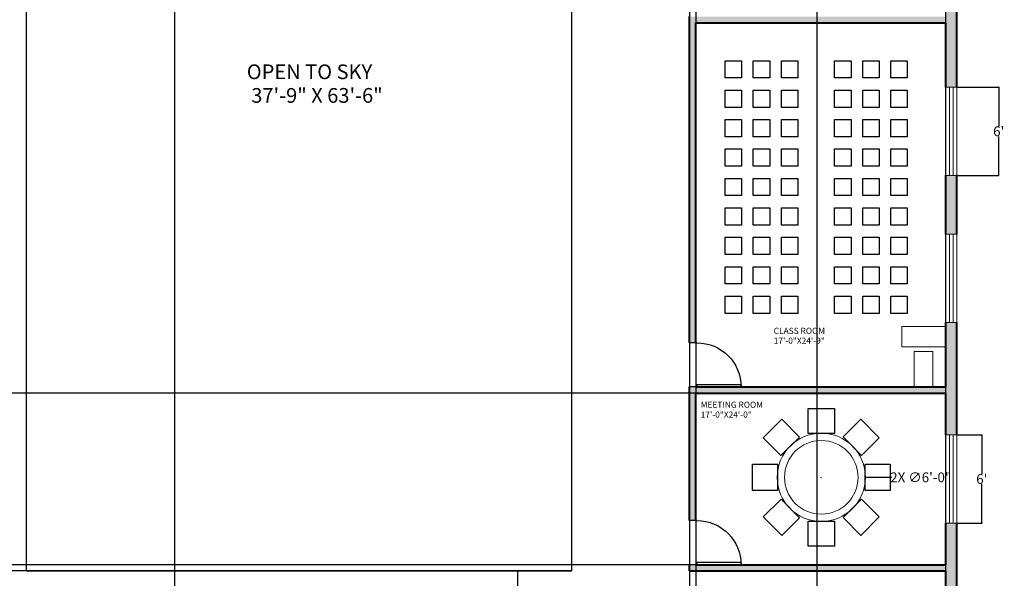
# Model space of a CAD drawing. Units: inches. Extents: x -405 to 940, y 226 to 2032.
# Tile 7 of 10: x 51 to 854, y 846 to 1301. Entities that reach past the tile are written whole.
import ezdxf

# ---------------------------------------------------------------- set-up
doc = ezdxf.new("R2010")
doc.units = ezdxf.units.IN
doc.header["$MEASUREMENT"] = 0
doc.linetypes.add('ACAD_ISO02W100', pattern=[15, 12, -3])
for name, color, linetype, lineweight in [('A-ANNO-DIMS', 120, 'Continuous', 18), ('A-AREA-IDEN', 32, 'Continuous', 18), ('A-FLOR-EDGE', 3, 'Continuous', 25), ('A-FURN-SEAT', 5, 'Continuous', 18), ('A-GLAZ-HIDN', 1, 'ACAD_ISO02W100', 18), ('A-WALL-PATT', 8, 'Continuous', 13), ('door', 6, 'Continuous', 25), ('tables', 2, 'Continuous', 18), ('wall', 3, 'Continuous', 40), ('window', 1, 'Continuous', 18)]:
    doc.layers.add(name, color=color, linetype=linetype, lineweight=lineweight)
doc.layers.add('beches', color=5, linetype='Continuous')
doc.styles.get("Standard").update_dxf_attribs({"font": 'arial.ttf'})
doc.dimstyles.get("Standard").update_dxf_attribs({"dimtxt": 8, "dimasz": 0.18, "dimexe": 0.18, "dimexo": 0.0625, "dimgap": 0.09, "dimtad": 0, "dimtih": 1, "dimtoh": 1, "dimdec": 0, "dimzin": 0, "dimdsep": 46, "dimlunit": 3, "dimtxsty": 'Standard', "dimblk": 'OBLIQUE', "dimcen": 0.09, "dimadec": 0, "dimazin": 0, "dimtfac": 1, "dimtdec": 0, "dimtofl": 0, "dimtmove": 0, "dimatfit": 3, "dimfxl": 1, "dimtolj": 1, "dimtzin": 0, "dimarcsym": 0})

# ---------------------------------------------------------------- blocks, each defined once
blk = doc.blocks.new('*U4')
for p, q in [((0, 0), (0, -6)), ((36, 0), (36, -6))]:
    blk.add_line(p, q)
blk.add_lwpolyline([(0, 0), (0, 36), (1.75, 36), (1.75, 0)], close=True)
blk.add_arc((0, 0), 36, 0, 90)
blk = doc.blocks.new('*U21')
at = {"layer": 'beches'}
blk.add_lwpolyline([(6.71, -7.02), (-6.71, -7.02), (-6.71, 7.02), (6.71, 7.02)], close=True, dxfattribs=at)
blk = doc.blocks.new('*U22')
at = {"layer": 'A-FURN-SEAT', "transparency": 16777216}
for p in [(-45.84, 192), (-45.84, 192, 12), (-45.84, 192, 24), (-45.84, 192, 36), (-45.84, 192, 48), (-45.84, 192, 60), (-45.84, 192, 72), (-45.84, 192, 84), (-45.84, 192, 96), (-45.84, 192, 108), (-45.84, 192, 120), (-45.84, 192, 132), (-22.92, 192), (-22.92, 192, 12), (-22.92, 192, 24), (-22.92, 192, 36), (-22.92, 192, 48), (-22.92, 192, 60), (-22.92, 192, 72), (-22.92, 192, 84), (-22.92, 192, 96), (-22.92, 192, 108), (-22.92, 192, 120), (-22.92, 192, 132), (0, 192), (0, 192, 12), (0, 192, 24), (0, 192, 36), (0, 192, 48), (0, 192, 60), (0, 192, 72), (0, 192, 84), (0, 192, 96), (0, 192, 108), (0, 192, 120), (0, 192, 132), (-45.84, 168), (-45.84, 168, 12), (-45.84, 168, 24), (-45.84, 168, 36), (-45.84, 168, 48), (-45.84, 168, 60), (-45.84, 168, 72), (-45.84, 168, 84), (-45.84, 168, 96), (-45.84, 168, 108), (-45.84, 168, 120), (-45.84, 168, 132), (-22.92, 168), (-22.92, 168, 12), (-22.92, 168, 24), (-22.92, 168, 36), (-22.92, 168, 48), (-22.92, 168, 60), (-22.92, 168, 72), (-22.92, 168, 84), (-22.92, 168, 96), (-22.92, 168, 108), (-22.92, 168, 120), (-22.92, 168, 132), (0, 168), (0, 168, 12), (0, 168, 24), (0, 168, 36), (0, 168, 48), (0, 168, 60), (0, 168, 72), (0, 168, 84), (0, 168, 96), (0, 168, 108), (0, 168, 120), (0, 168, 132), (-45.84, 144), (-45.84, 144, 12), (-45.84, 144, 24), (-45.84, 144, 36), (-45.84, 144, 48), (-45.84, 144, 60), (-45.84, 144, 72), (-45.84, 144, 84), (-45.84, 144, 96), (-45.84, 144, 108), (-45.84, 144, 120), (-45.84, 144, 132), (-22.92, 144), (-22.92, 144, 12), (-22.92, 144, 24), (-22.92, 144, 36), (-22.92, 144, 48), (-22.92, 144, 60), (-22.92, 144, 72), (-22.92, 144, 84), (-22.92, 144, 96), (-22.92, 144, 108), (-22.92, 144, 120), (-22.92, 144, 132), (0, 144), (0, 144, 12), (0, 144, 24), (0, 144, 36), (0, 144, 48), (0, 144, 60), (0, 144, 72), (0, 144, 84), (0, 144, 96), (0, 144, 108), (0, 144, 120), (0, 144, 132), (-45.84, 120), (-45.84, 120, 12), (-45.84, 120, 24), (-45.84, 120, 36), (-45.84, 120, 48), (-45.84, 120, 60), (-45.84, 120, 72), (-45.84, 120, 84), (-45.84, 120, 96), (-45.84, 120, 108), (-45.84, 120, 120), (-45.84, 120, 132), (-22.92, 120), (-22.92, 120, 12), (-22.92, 120, 24), (-22.92, 120, 36), (-22.92, 120, 48), (-22.92, 120, 60), (-22.92, 120, 72), (-22.92, 120, 84), (-22.92, 120, 96), (-22.92, 120, 108), (-22.92, 120, 120), (-22.92, 120, 132), (0, 120), (0, 120, 12), (0, 120, 24), (0, 120, 36), (0, 120, 48), (0, 120, 60), (0, 120, 72), (0, 120, 84), (0, 120, 96), (0, 120, 108), (0, 120, 120), (0, 120, 132), (-45.84, 96), (-45.84, 96, 12), (-45.84, 96, 24), (-45.84, 96, 36), (-45.84, 96, 48), (-45.84, 96, 60), (-45.84, 96, 72), (-45.84, 96, 84), (-45.84, 96, 96), (-45.84, 96, 108), (-45.84, 96, 120), (-45.84, 96, 132), (-22.92, 96), (-22.92, 96, 12), (-22.92, 96, 24), (-22.92, 96, 36), (-22.92, 96, 48), (-22.92, 96, 60), (-22.92, 96, 72), (-22.92, 96, 84), (-22.92, 96, 96), (-22.92, 96, 108), (-22.92, 96, 120), (-22.92, 96, 132), (0, 96), (0, 96, 12), (0, 96, 24), (0, 96, 36), (0, 96, 48), (0, 96, 60), (0, 96, 72), (0, 96, 84), (0, 96, 96), (0, 96, 108), (0, 96, 120), (0, 96, 132), (-45.84, 72), (-45.84, 72, 12), (-45.84, 72, 24), (-45.84, 72, 36), (-45.84, 72, 48), (-45.84, 72, 60), (-45.84, 72, 72), (-45.84, 72, 84), (-45.84, 72, 96), (-45.84, 72, 108), (-45.84, 72, 120), (-45.84, 72, 132), (-22.92, 72), (-22.92, 72, 12), (-22.92, 72, 24), (-22.92, 72, 36), (-22.92, 72, 48), (-22.92, 72, 60), (-22.92, 72, 72), (-22.92, 72, 84), (-22.92, 72, 96), (-22.92, 72, 108), (-22.92, 72, 120), (-22.92, 72, 132), (0, 72), (0, 72, 12), (0, 72, 24), (0, 72, 36), (0, 72, 48), (0, 72, 60), (0, 72, 72), (0, 72, 84), (0, 72, 96), (0, 72, 108), (0, 72, 120), (0, 72, 132), (-45.84, 48), (-45.84, 48, 12), (-45.84, 48, 24), (-45.84, 48, 36), (-45.84, 48, 48), (-45.84, 48, 60), (-45.84, 48, 72), (-45.84, 48, 84), (-45.84, 48, 96), (-45.84, 48, 108), (-45.84, 48, 120), (-45.84, 48, 132), (-22.92, 48), (-22.92, 48, 12), (-22.92, 48, 24), (-22.92, 48, 36), (-22.92, 48, 48), (-22.92, 48, 60), (-22.92, 48, 72), (-22.92, 48, 84), (-22.92, 48, 96), (-22.92, 48, 108), (-22.92, 48, 120), (-22.92, 48, 132), (0, 48), (0, 48, 12), (0, 48, 24), (0, 48, 36), (0, 48, 48), (0, 48, 60), (0, 48, 72), (0, 48, 84), (0, 48, 96), (0, 48, 108), (0, 48, 120), (0, 48, 132), (-45.84, 24), (-45.84, 24, 12), (-45.84, 24, 24), (-45.84, 24, 36), (-45.84, 24, 48), (-45.84, 24, 60), (-45.84, 24, 72), (-45.84, 24, 84), (-45.84, 24, 96), (-45.84, 24, 108), (-45.84, 24, 120), (-45.84, 24, 132), (-22.92, 24), (-22.92, 24, 12), (-22.92, 24, 24), (-22.92, 24, 36), (-22.92, 24, 48), (-22.92, 24, 60), (-22.92, 24, 72), (-22.92, 24, 84), (-22.92, 24, 96), (-22.92, 24, 108), (-22.92, 24, 120), (-22.92, 24, 132), (0, 24), (0, 24, 12), (0, 24, 24), (0, 24, 36), (0, 24, 48), (0, 24, 60), (0, 24, 72), (0, 24, 84), (0, 24, 96), (0, 24, 108), (0, 24, 120), (0, 24, 132), (-45.84, 0), (-45.84, 0, 12), (-45.84, 0, 24), (-45.84, 0, 36), (-45.84, 0, 48), (-45.84, 0, 60), (-45.84, 0, 72), (-45.84, 0, 84), (-45.84, 0, 96), (-45.84, 0, 108), (-45.84, 0, 120), (-45.84, 0, 132), (-22.92, 0), (-22.92, 0, 12), (-22.92, 0, 24), (-22.92, 0, 36), (-22.92, 0, 48), (-22.92, 0, 60), (-22.92, 0, 72), (-22.92, 0, 84), (-22.92, 0, 96), (-22.92, 0, 108), (-22.92, 0, 120), (-22.92, 0, 132), (0, 0), (0, 0, 12), (0, 0, 24), (0, 0, 36), (0, 0, 48), (0, 0, 60), (0, 0, 72), (0, 0, 84), (0, 0, 96), (0, 0, 108), (0, 0, 120), (0, 0, 132)]:
    blk.add_blockref('*U21', p, dxfattribs=at)
blk = doc.blocks.new('*U19')
at = {"layer": 'beches'}
blk.add_lwpolyline([(6.71, -7.02), (-6.71, -7.02), (-6.71, 7.02), (6.71, 7.02)], close=True, dxfattribs=at)
blk = doc.blocks.new('*U20')
at = {"layer": 'A-FURN-SEAT', "transparency": 16777216}
for p in [(-45.84, 192), (-45.84, 192, 12), (-45.84, 192, 24), (-45.84, 192, 36), (-45.84, 192, 48), (-45.84, 192, 60), (-45.84, 192, 72), (-45.84, 192, 84), (-45.84, 192, 96), (-45.84, 192, 108), (-45.84, 192, 120), (-45.84, 192, 132), (-22.92, 192), (-22.92, 192, 12), (-22.92, 192, 24), (-22.92, 192, 36), (-22.92, 192, 48), (-22.92, 192, 60), (-22.92, 192, 72), (-22.92, 192, 84), (-22.92, 192, 96), (-22.92, 192, 108), (-22.92, 192, 120), (-22.92, 192, 132), (0, 192), (0, 192, 12), (0, 192, 24), (0, 192, 36), (0, 192, 48), (0, 192, 60), (0, 192, 72), (0, 192, 84), (0, 192, 96), (0, 192, 108), (0, 192, 120), (0, 192, 132), (-45.84, 168), (-45.84, 168, 12), (-45.84, 168, 24), (-45.84, 168, 36), (-45.84, 168, 48), (-45.84, 168, 60), (-45.84, 168, 72), (-45.84, 168, 84), (-45.84, 168, 96), (-45.84, 168, 108), (-45.84, 168, 120), (-45.84, 168, 132), (-22.92, 168), (-22.92, 168, 12), (-22.92, 168, 24), (-22.92, 168, 36), (-22.92, 168, 48), (-22.92, 168, 60), (-22.92, 168, 72), (-22.92, 168, 84), (-22.92, 168, 96), (-22.92, 168, 108), (-22.92, 168, 120), (-22.92, 168, 132), (0, 168), (0, 168, 12), (0, 168, 24), (0, 168, 36), (0, 168, 48), (0, 168, 60), (0, 168, 72), (0, 168, 84), (0, 168, 96), (0, 168, 108), (0, 168, 120), (0, 168, 132), (-45.84, 144), (-45.84, 144, 12), (-45.84, 144, 24), (-45.84, 144, 36), (-45.84, 144, 48), (-45.84, 144, 60), (-45.84, 144, 72), (-45.84, 144, 84), (-45.84, 144, 96), (-45.84, 144, 108), (-45.84, 144, 120), (-45.84, 144, 132), (-22.92, 144), (-22.92, 144, 12), (-22.92, 144, 24), (-22.92, 144, 36), (-22.92, 144, 48), (-22.92, 144, 60), (-22.92, 144, 72), (-22.92, 144, 84), (-22.92, 144, 96), (-22.92, 144, 108), (-22.92, 144, 120), (-22.92, 144, 132), (0, 144), (0, 144, 12), (0, 144, 24), (0, 144, 36), (0, 144, 48), (0, 144, 60), (0, 144, 72), (0, 144, 84), (0, 144, 96), (0, 144, 108), (0, 144, 120), (0, 144, 132), (-45.84, 120), (-45.84, 120, 12), (-45.84, 120, 24), (-45.84, 120, 36), (-45.84, 120, 48), (-45.84, 120, 60), (-45.84, 120, 72), (-45.84, 120, 84), (-45.84, 120, 96), (-45.84, 120, 108), (-45.84, 120, 120), (-45.84, 120, 132), (-22.92, 120), (-22.92, 120, 12), (-22.92, 120, 24), (-22.92, 120, 36), (-22.92, 120, 48), (-22.92, 120, 60), (-22.92, 120, 72), (-22.92, 120, 84), (-22.92, 120, 96), (-22.92, 120, 108), (-22.92, 120, 120), (-22.92, 120, 132), (0, 120), (0, 120, 12), (0, 120, 24), (0, 120, 36), (0, 120, 48), (0, 120, 60), (0, 120, 72), (0, 120, 84), (0, 120, 96), (0, 120, 108), (0, 120, 120), (0, 120, 132), (-45.84, 96), (-45.84, 96, 12), (-45.84, 96, 24), (-45.84, 96, 36), (-45.84, 96, 48), (-45.84, 96, 60), (-45.84, 96, 72), (-45.84, 96, 84), (-45.84, 96, 96), (-45.84, 96, 108), (-45.84, 96, 120), (-45.84, 96, 132), (-22.92, 96), (-22.92, 96, 12), (-22.92, 96, 24), (-22.92, 96, 36), (-22.92, 96, 48), (-22.92, 96, 60), (-22.92, 96, 72), (-22.92, 96, 84), (-22.92, 96, 96), (-22.92, 96, 108), (-22.92, 96, 120), (-22.92, 96, 132), (0, 96), (0, 96, 12), (0, 96, 24), (0, 96, 36), (0, 96, 48), (0, 96, 60), (0, 96, 72), (0, 96, 84), (0, 96, 96), (0, 96, 108), (0, 96, 120), (0, 96, 132), (-45.84, 72), (-45.84, 72, 12), (-45.84, 72, 24), (-45.84, 72, 36), (-45.84, 72, 48), (-45.84, 72, 60), (-45.84, 72, 72), (-45.84, 72, 84), (-45.84, 72, 96), (-45.84, 72, 108), (-45.84, 72, 120), (-45.84, 72, 132), (-22.92, 72), (-22.92, 72, 12), (-22.92, 72, 24), (-22.92, 72, 36), (-22.92, 72, 48), (-22.92, 72, 60), (-22.92, 72, 72), (-22.92, 72, 84), (-22.92, 72, 96), (-22.92, 72, 108), (-22.92, 72, 120), (-22.92, 72, 132), (0, 72), (0, 72, 12), (0, 72, 24), (0, 72, 36), (0, 72, 48), (0, 72, 60), (0, 72, 72), (0, 72, 84), (0, 72, 96), (0, 72, 108), (0, 72, 120), (0, 72, 132), (-45.84, 48), (-45.84, 48, 12), (-45.84, 48, 24), (-45.84, 48, 36), (-45.84, 48, 48), (-45.84, 48, 60), (-45.84, 48, 72), (-45.84, 48, 84), (-45.84, 48, 96), (-45.84, 48, 108), (-45.84, 48, 120), (-45.84, 48, 132), (-22.92, 48), (-22.92, 48, 12), (-22.92, 48, 24), (-22.92, 48, 36), (-22.92, 48, 48), (-22.92, 48, 60), (-22.92, 48, 72), (-22.92, 48, 84), (-22.92, 48, 96), (-22.92, 48, 108), (-22.92, 48, 120), (-22.92, 48, 132), (0, 48), (0, 48, 12), (0, 48, 24), (0, 48, 36), (0, 48, 48), (0, 48, 60), (0, 48, 72), (0, 48, 84), (0, 48, 96), (0, 48, 108), (0, 48, 120), (0, 48, 132), (-45.84, 24), (-45.84, 24, 12), (-45.84, 24, 24), (-45.84, 24, 36), (-45.84, 24, 48), (-45.84, 24, 60), (-45.84, 24, 72), (-45.84, 24, 84), (-45.84, 24, 96), (-45.84, 24, 108), (-45.84, 24, 120), (-45.84, 24, 132), (-22.92, 24), (-22.92, 24, 12), (-22.92, 24, 24), (-22.92, 24, 36), (-22.92, 24, 48), (-22.92, 24, 60), (-22.92, 24, 72), (-22.92, 24, 84), (-22.92, 24, 96), (-22.92, 24, 108), (-22.92, 24, 120), (-22.92, 24, 132), (0, 24), (0, 24, 12), (0, 24, 24), (0, 24, 36), (0, 24, 48), (0, 24, 60), (0, 24, 72), (0, 24, 84), (0, 24, 96), (0, 24, 108), (0, 24, 120), (0, 24, 132), (-45.84, 0), (-45.84, 0, 12), (-45.84, 0, 24), (-45.84, 0, 36), (-45.84, 0, 48), (-45.84, 0, 60), (-45.84, 0, 72), (-45.84, 0, 84), (-45.84, 0, 96), (-45.84, 0, 108), (-45.84, 0, 120), (-45.84, 0, 132), (-22.92, 0), (-22.92, 0, 12), (-22.92, 0, 24), (-22.92, 0, 36), (-22.92, 0, 48), (-22.92, 0, 60), (-22.92, 0, 72), (-22.92, 0, 84), (-22.92, 0, 96), (-22.92, 0, 108), (-22.92, 0, 120), (-22.92, 0, 132), (0, 0), (0, 0, 12), (0, 0, 24), (0, 0, 36), (0, 0, 48), (0, 0, 60), (0, 0, 72), (0, 0, 84), (0, 0, 96), (0, 0, 108), (0, 0, 120), (0, 0, 132)]:
    blk.add_blockref('*U19', p, dxfattribs=at)
blk = doc.blocks.new('*U37')
at = {"layer": 'beches'}
blk.add_lwpolyline([(-10.7, 10.22), (10.7, 10.22), (10.7, -10.22), (-10.7, -10.22)], close=True, dxfattribs=at)
blk = doc.blocks.new('*U38')
at = {"layer": 'A-FURN-SEAT', "transparency": 16777216}
blk.add_blockref('*U37', (125.75, 1834.83), dxfattribs=at)
for p, rotation in [((93.21, 1821.33), 45.00000000000002), ((158.29, 1821.37), 314.9999999999999), ((79.75, 1788.79), 90.00000000000003), ((171.79, 1788.83), 270), ((93.24, 1756.26), 135), ((158.32, 1756.29), 225), ((125.79, 1742.79), 180)]:
    blk.add_blockref('*U37', p, dxfattribs=dict(at, rotation=rotation))
blk = doc.blocks.new('_Oblique')
at = {"color": 0, "linetype": 'ByBlock', "lineweight": -2}
blk.add_line((-0.5, -0.5), (0.5, 0.5), dxfattribs=at)
blk = doc.blocks.new('*D39')
at = {"layer": 'A-ANNO-DIMS', "color": 0, "lineweight": -2, "transparency": 16777216}
for p, q in [((460.94, 851.81), (457.18, 851.81)), ((457.36, 851.81), (457.36, 807.98)), ((457.36, 755.81), (457.36, 799.64)), ((460.94, 755.81), (457.18, 755.81))]:
    blk.add_line(p, q, dxfattribs=at)
at = {"layer": 'Defpoints', "color": 0, "transparency": 16777216}
for p in [(457.36, 851.81), (461, 851.81), (461, 755.81)]:
    blk.add_point(p, dxfattribs=at)
at = {"layer": 'A-ANNO-DIMS', "color": 0, "lineweight": -2, "transparency": 16777216, "xscale": 0.18, "yscale": 0.18, "zscale": 0.18}
for p, rotation in [((457.36, 851.81), 90), ((457.36, 755.81), 270)]:
    blk.add_blockref('_Oblique', p, dxfattribs=dict(at, rotation=rotation))
at = {"layer": 'A-ANNO-DIMS', "color": 0, "transparency": 16777216, "insert": (457.36, 803.81), "char_height": 8, "attachment_point": 5}
blk.add_mtext("\\A1;8'", dxfattribs=at)
blk = doc.blocks.new('*D70')
at = {"layer": 'A-ANNO-DIMS', "color": 0, "lineweight": -2, "transparency": 16777216}
for p, q in [((815.83, 1246.31), (850.12, 1246.31)), ((849.94, 1246.31), (849.94, 1214.48)), ((849.94, 1174.31), (849.94, 1206.14)), ((815.83, 1174.31), (850.12, 1174.31))]:
    blk.add_line(p, q, dxfattribs=at)
at = {"layer": 'Defpoints', "color": 0, "transparency": 16777216}
for p in [(815.77, 1246.31), (815.77, 1174.31), (849.94, 1174.31)]:
    blk.add_point(p, dxfattribs=at)
at = {"layer": 'A-ANNO-DIMS', "color": 0, "lineweight": -2, "transparency": 16777216, "xscale": 0.18, "yscale": 0.18, "zscale": 0.18}
for p, rotation in [((849.94, 1246.31), 90), ((849.94, 1174.31), 270)]:
    blk.add_blockref('_Oblique', p, dxfattribs=dict(at, rotation=rotation))
at = {"layer": 'A-ANNO-DIMS', "color": 0, "transparency": 16777216, "insert": (849.94, 1210.31), "char_height": 8, "attachment_point": 5}
blk.add_mtext("\\A1;6'", dxfattribs=at)
blk = doc.blocks.new('*D71')
at = {"layer": 'A-ANNO-DIMS', "color": 0, "lineweight": -2, "transparency": 16777216}
for p, q in [((815.83, 962.81), (836.29, 962.81)), ((836.11, 962.81), (836.11, 930.98)), ((836.11, 890.81), (836.11, 922.64)), ((815.83, 890.81), (836.29, 890.81))]:
    blk.add_line(p, q, dxfattribs=at)
at = {"layer": 'Defpoints', "color": 0, "transparency": 16777216}
for p in [(815.77, 962.81), (815.77, 890.81), (836.11, 890.81)]:
    blk.add_point(p, dxfattribs=at)
at = {"layer": 'A-ANNO-DIMS', "color": 0, "lineweight": -2, "transparency": 16777216, "xscale": 0.18, "yscale": 0.18, "zscale": 0.18}
for p, rotation in [((836.11, 962.81), 90), ((836.11, 890.81), 270)]:
    blk.add_blockref('_Oblique', p, dxfattribs=dict(at, rotation=rotation))
at = {"layer": 'A-ANNO-DIMS', "color": 0, "transparency": 16777216, "insert": (836.11, 926.81), "char_height": 8, "attachment_point": 5}
blk.add_mtext("\\A1;6'", dxfattribs=at)
blk = doc.blocks.new('TABLE-ROUND-72IN')
for radius in [36, 30]:
    blk.add_circle((36, 36), radius)
blk = doc.blocks.new('CLASSROOM-DESK-WIDE')
for p, q in [((0, 0), (0, 16.56)), ((0, 16.56), (36, 16.56)), ((36, 16.56), (36, 0)), ((36, 0), (0, 0))]:
    blk.add_line(p, q)
blk = doc.blocks.new('WIN-PANE-72IN')
for p, q in [((0, 3), (72, 3)), ((0, 0), (72, 0))]:
    blk.add_line(p, q)
blk = doc.blocks.new('*D106')
at = {"layer": 'A-ANNO-DIMS', "color": 0, "lineweight": -2, "transparency": 16777216}
for p, q in [((56.77, 851.87), (56.77, 2020.64)), ((56.77, 2020.46), (265.44, 2020.46)), ((501.77, 2020.46), (293.1, 2020.46)), ((501.77, 851.87), (501.77, 2020.64))]:
    blk.add_line(p, q, dxfattribs=at)
at = {"layer": 'Defpoints', "color": 0, "transparency": 16777216}
for p in [(501.77, 2020.46), (56.77, 851.81), (501.77, 851.81)]:
    blk.add_point(p, dxfattribs=at)
at = {"layer": 'A-ANNO-DIMS', "color": 0, "lineweight": -2, "transparency": 16777216, "xscale": 0.18, "yscale": 0.18, "zscale": 0.18, "rotation": 180}
blk.add_blockref('_Oblique', (56.77, 2020.46), dxfattribs=at)
at = {"layer": 'A-ANNO-DIMS', "color": 0, "lineweight": -2, "transparency": 16777216, "xscale": 0.18, "yscale": 0.18, "zscale": 0.18}
blk.add_blockref('_Oblique', (501.77, 2020.46), dxfattribs=at)
at = {"layer": 'A-ANNO-DIMS', "color": 0, "transparency": 16777216, "insert": (279.27, 2020.46), "char_height": 8, "attachment_point": 5}
blk.add_mtext('\\A1;37\'-1"', dxfattribs=at)
blk = doc.blocks.new('*D107')
at = {"layer": 'A-ANNO-DIMS', "color": 0, "lineweight": -2, "transparency": 16777216}
for p, q in [((501.71, 1597.81), (-390.06, 1597.81)), ((-389.88, 1597.81), (-389.88, 1228.98)), ((-389.88, 851.81), (-389.88, 1220.64)), ((501.71, 851.81), (-390.06, 851.81))]:
    blk.add_line(p, q, dxfattribs=at)
at = {"layer": 'Defpoints', "color": 0, "transparency": 16777216}
for p in [(-389.88, 1597.81), (501.77, 1597.81), (501.77, 851.81)]:
    blk.add_point(p, dxfattribs=at)
at = {"layer": 'A-ANNO-DIMS', "color": 0, "lineweight": -2, "transparency": 16777216, "xscale": 0.18, "yscale": 0.18, "zscale": 0.18}
for p, rotation in [((-389.88, 1597.81), 90), ((-389.88, 851.81), 270)]:
    blk.add_blockref('_Oblique', p, dxfattribs=dict(at, rotation=rotation))
at = {"layer": 'A-ANNO-DIMS', "color": 0, "transparency": 16777216, "insert": (-389.88, 1224.81), "char_height": 8, "attachment_point": 5}
blk.add_mtext('\\A1;62\'-2"', dxfattribs=at)
blk = doc.blocks.new('*D108')
at = {"layer": 'A-ANNO-DIMS', "color": 0, "lineweight": -2, "transparency": 16777216}
for p, q in [((806.71, 996.81), (-390.06, 996.81)), ((-389.88, 996.81), (-389.88, 930.98)), ((-389.88, 856.81), (-389.88, 922.64)), ((806.71, 856.81), (-390.06, 856.81))]:
    blk.add_line(p, q, dxfattribs=at)
at = {"layer": 'Defpoints', "color": 0, "transparency": 16777216}
for p in [(-389.88, 996.81), (806.77, 996.81), (806.77, 856.81)]:
    blk.add_point(p, dxfattribs=at)
at = {"layer": 'A-ANNO-DIMS', "color": 0, "lineweight": -2, "transparency": 16777216, "xscale": 0.18, "yscale": 0.18, "zscale": 0.18}
for p, rotation in [((-389.88, 996.81), 90), ((-389.88, 856.81), 270)]:
    blk.add_blockref('_Oblique', p, dxfattribs=dict(at, rotation=rotation))
at = {"layer": 'A-ANNO-DIMS', "color": 0, "transparency": 16777216, "insert": (-389.88, 926.81), "char_height": 8, "attachment_point": 5}
blk.add_mtext('\\A1;11\'-8"', dxfattribs=at)
blk = doc.blocks.new('*D109')
at = {"layer": 'A-ANNO-DIMS', "color": 0, "lineweight": -2, "transparency": 16777216}
for p, q in [((-248.23, 750.87), (-248.23, 2020.64)), ((-248.23, 2020.46), (-49.06, 2020.46)), ((177.77, 2020.46), (-21.4, 2020.46)), ((177.77, 750.87), (177.77, 2020.64))]:
    blk.add_line(p, q, dxfattribs=at)
at = {"layer": 'Defpoints', "color": 0, "transparency": 16777216}
for p in [(177.77, 2020.46), (-248.23, 750.81), (177.77, 750.81)]:
    blk.add_point(p, dxfattribs=at)
at = {"layer": 'A-ANNO-DIMS', "color": 0, "lineweight": -2, "transparency": 16777216, "xscale": 0.18, "yscale": 0.18, "zscale": 0.18, "rotation": 180}
blk.add_blockref('_Oblique', (-248.23, 2020.46), dxfattribs=at)
at = {"layer": 'A-ANNO-DIMS', "color": 0, "lineweight": -2, "transparency": 16777216, "xscale": 0.18, "yscale": 0.18, "zscale": 0.18}
blk.add_blockref('_Oblique', (177.77, 2020.46), dxfattribs=at)
at = {"layer": 'A-ANNO-DIMS', "color": 0, "transparency": 16777216, "insert": (-35.23, 2020.46), "char_height": 8, "attachment_point": 5}
blk.add_mtext('\\A1;35\'-6"', dxfattribs=at)
blk = doc.blocks.new('*D112')
at = {"layer": 'A-ANNO-DIMS', "color": 0, "lineweight": -2, "transparency": 16777216}
for p, q in [((701.77, 534.87), (701.77, 2020.64)), ((701.77, 2020.46), (743.54, 2020.46)), ((806.77, 2020.46), (765, 2020.46)), ((806.77, 534.87), (806.77, 2020.64))]:
    blk.add_line(p, q, dxfattribs=at)
at = {"layer": 'Defpoints', "color": 0, "transparency": 16777216}
for p in [(701.77, 2020.46), (701.77, 534.81), (806.77, 534.81)]:
    blk.add_point(p, dxfattribs=at)
at = {"layer": 'A-ANNO-DIMS', "color": 0, "lineweight": -2, "transparency": 16777216, "xscale": 0.18, "yscale": 0.18, "zscale": 0.18, "rotation": 180}
blk.add_blockref('_Oblique', (701.77, 2020.46), dxfattribs=at)
at = {"layer": 'A-ANNO-DIMS', "color": 0, "lineweight": -2, "transparency": 16777216, "xscale": 0.18, "yscale": 0.18, "zscale": 0.18}
blk.add_blockref('_Oblique', (806.77, 2020.46), dxfattribs=at)
at = {"layer": 'A-ANNO-DIMS', "color": 0, "transparency": 16777216, "insert": (754.27, 2020.46), "char_height": 8, "attachment_point": 5}
blk.add_mtext('\\A1;8\'-9"', dxfattribs=at)
blk = doc.blocks.new('*D116')
at = {"layer": 'A-ANNO-DIMS', "color": 0, "lineweight": -2, "transparency": 16777216}
for p, q in [((597.77, 1339.75), (597.77, 230.98)), ((602.77, 1339.75), (602.77, 230.98)), ((597.77, 231.16), (602.77, 231.16)), ((602.77, 231.16), (602.95, 231.16))]:
    blk.add_line(p, q, dxfattribs=at)
at = {"layer": 'Defpoints', "color": 0, "transparency": 16777216}
for p in [(597.77, 1339.81), (602.77, 1339.81), (602.77, 231.16)]:
    blk.add_point(p, dxfattribs=at)
at = {"layer": 'A-ANNO-DIMS', "color": 0, "lineweight": -2, "transparency": 16777216, "xscale": 0.18, "yscale": 0.18, "zscale": 0.18, "rotation": 180}
blk.add_blockref('_Oblique', (597.77, 231.16), dxfattribs=at)
at = {"layer": 'A-ANNO-DIMS', "color": 0, "lineweight": -2, "transparency": 16777216, "xscale": 0.18, "yscale": 0.18, "zscale": 0.18}
blk.add_blockref('_Oblique', (602.77, 231.16), dxfattribs=at)
at = {"layer": 'A-ANNO-DIMS', "color": 0, "transparency": 16777216, "insert": (613.67, 231.16), "char_height": 8, "attachment_point": 5}
blk.add_mtext('\\A1;0\'-5"', dxfattribs=at)
blk = doc.blocks.new('*D117')
at = {"layer": 'A-ANNO-DIMS', "color": 0, "lineweight": -2, "transparency": 16777216}
for p, q in [((705.1, 928.12), (705.28, 928.12)), ((705.19, 928.03), (705.19, 928.21)), ((762.79, 928.12), (741.19, 928.12))]:
    blk.add_line(p, q, dxfattribs=at)
at = {"layer": 'Defpoints', "color": 0, "transparency": 16777216}
for p in [(669.19, 928.12), (741.19, 928.12)]:
    blk.add_point(p, dxfattribs=at)
at = {"layer": 'A-ANNO-DIMS', "color": 0, "lineweight": -2, "transparency": 16777216, "xscale": 0.18, "yscale": 0.18, "zscale": 0.18, "rotation": 179.9994763802373}
blk.add_blockref('_Oblique', (741.19, 928.12), dxfattribs=at)
at = {"layer": 'A-ANNO-DIMS', "color": 0, "transparency": 16777216, "insert": (786.32, 928.12), "char_height": 8, "attachment_point": 5}
blk.add_mtext('\\A1;2X ∅6\'-0"', dxfattribs=at)

msp = doc.modelspace()

# ---------------------------------------------------------------- hatches: boundary and pattern name
at = {"layer": 'A-WALL-PATT'}
h = msp.add_hatch(dxfattribs=at)
h.set_pattern_fill('AR-HBONE', color=256)
h.set_pattern_definition([(45, (599.8442, 904.9158), (0, 5.656854), [12, -4]), (135, (602.6726, 907.744), (4e-16, 5.656854), [12, -4])])
h.paths.add_polyline_path([(-248.23, 1045.81), (-257.23, 1045.81), (-257.23, 964.81), (-248.23, 964.81)], flags=17)
h.paths.add_polyline_path([(-248.23, 851.81), (-39.23, 851.81), (-39.23, 856.81), (-44.23, 856.81), (-248.23, 856.81), (-248.23, 892.81), (-257.23, 892.81), (-257.23, 839.81), (-248.23, 839.81)])
h.paths.add_polyline_path([(-248.23, 750.81), (124.74, 750.81), (124.74, 751.73), (124.74, 755.81), (-248.23, 755.81), (-248.23, 767.81), (-257.23, 767.81), (-257.23, 726.81), (-248.23, 726.81)])
h.paths.add_polyline_path([(-248.23, 654.81), (-257.23, 654.81), (-257.23, 630.81), (-248.23, 630.81)])
h.paths.add_polyline_path([(-180.23, 534.81), (-248.23, 534.81), (-248.23, 558.81), (-257.23, 558.81), (-257.23, 525.81), (-180.23, 525.81)])
h.paths.add_polyline_path([(-69.23, 534.81), (-108.23, 534.81), (-108.23, 525.81), (-69.23, 525.81)])
h.paths.add_polyline_path([(35.77, 534.81), (2.77, 534.81), (2.77, 525.81), (35.77, 525.81)])
h.paths.add_polyline_path([(182.77, 755.81), (160.74, 755.81), (160.74, 750.81), (177.77, 750.81), (177.77, 534.81), (107.77, 534.81), (107.77, 525.81), (182.77, 525.81)])
h.paths.add_polyline_path([(-39.23, 1609.81), (-44.23, 1609.81), (-44.23, 1604.81), (-44.23, 1460.81), (-135.23, 1460.81), (-135.23, 1465.73), (-140.23, 1465.73), (-140.23, 1460.81), (-248.23, 1460.81), (-248.23, 1471.31), (-257.23, 1471.31), (-257.23, 1419.81), (-248.23, 1419.81), (-248.23, 1455.81), (-44.23, 1455.81), (-44.23, 1194.81), (-39.23, 1194.81)])
h.paths.add_polyline_path([(-248.23, 1520.81), (-257.23, 1520.81), (-257.23, 1495.31), (-248.23, 1495.31), (-248.23, 1505.81), (-140.23, 1505.81), (-140.23, 1495.73), (-135.23, 1495.73), (-135.23, 1516.79), (-140.23, 1516.79), (-140.23, 1510.81), (-248.23, 1510.81)], flags=17)
h.paths.add_polyline_path([(-248.23, 1570.31), (-257.23, 1570.31), (-257.23, 1544.81), (-248.23, 1544.81), (-248.23, 1554.81), (-140.23, 1554.81), (-140.23, 1546.79), (-135.23, 1546.79), (-135.23, 1565.08), (-140.23, 1565.08), (-140.23, 1559.81), (-248.23, 1559.81)], flags=17)
h.paths.add_polyline_path([(-248.23, 1615.81), (-257.23, 1615.81), (-257.23, 1594.31), (-248.23, 1594.31), (-248.23, 1604.81), (-140.23, 1604.81), (-140.23, 1595.08), (-135.23, 1595.08), (-135.23, 1604.81), (-80.23, 1604.81), (-80.23, 1609.81), (-248.23, 1609.81)])
h.paths.add_polyline_path([(-248.23, 1783.81), (-235.46, 1783.81), (-235.46, 1788.81), (-248.23, 1788.81), (-248.23, 1878.81), (-237.73, 1878.81), (-237.73, 1887.81), (-257.23, 1887.81), (-257.23, 1687.81), (-248.23, 1687.81), (-248.23, 1693.81), (-136.23, 1693.81), (-136.23, 1698.81), (-248.23, 1698.81)])
h.paths.add_polyline_path([(-188.23, 1887.81), (-213.73, 1887.81), (-213.73, 1878.81), (-203.23, 1878.81), (-203.23, 1788.81), (-205.46, 1788.81), (-205.46, 1783.81), (-186.39, 1783.81), (-186.39, 1788.81), (-198.23, 1788.81), (-198.23, 1878.81), (-188.23, 1878.81)])
h.paths.add_polyline_path([(-139.23, 1887.81), (-164.23, 1887.81), (-164.23, 1878.81), (-154.23, 1878.81), (-154.23, 1788.81), (-156.39, 1788.81), (-156.39, 1783.81), (-138.25, 1783.81), (-138.25, 1788.81), (-149.23, 1788.81), (-149.23, 1878.81), (-139.23, 1878.81)])
h.paths.add_polyline_path([(-89.23, 1887.81), (-115.23, 1887.81), (-115.23, 1878.81), (-105.23, 1878.81), (-105.23, 1788.81), (-108.25, 1788.81), (-108.25, 1783.81), (-86.45, 1783.81), (-86.45, 1788.81), (-100.23, 1788.81), (-100.23, 1878.81), (-89.23, 1878.81)])
h.paths.add_polyline_path([(-36.23, 1887.81), (-65.23, 1887.81), (-65.23, 1878.81), (-54.23, 1878.81), (-54.23, 1788.81), (-56.45, 1788.81), (-56.45, 1783.81), (-54.23, 1783.81), (-54.23, 1698.81), (-100.23, 1698.81), (-100.23, 1693.81), (-49.23, 1693.81), (-49.23, 1698.81), (-49.23, 1878.81), (-36.23, 1878.81)])
h.paths.add_polyline_path([(89.77, 1887.81), (35.77, 1887.81), (35.77, 1878.81), (48.77, 1878.81), (48.77, 1698.81), (-13.23, 1698.81), (-13.23, 1693.81), (53.77, 1693.81), (53.77, 1698.81), (53.77, 1878.81), (89.77, 1878.81)])
h.paths.add_polyline_path([(255.27, 1887.81), (161.77, 1887.81), (161.77, 1878.81), (197.77, 1878.81), (197.77, 1698.81), (89.77, 1698.81), (89.77, 1693.81), (202.77, 1693.81), (202.77, 1698.81), (202.77, 1878.81), (255.27, 1878.81)])
h.paths.add_polyline_path([(375.27, 1887.81), (327.27, 1887.81), (327.27, 1878.81), (375.27, 1878.81)], flags=17)
h.paths.add_polyline_path([(815.77, 1887.81), (447.27, 1887.81), (447.27, 1878.81), (499.77, 1878.81), (499.77, 1698.81), (238.77, 1698.81), (238.77, 1693.81), (504.77, 1693.81), (504.77, 1878.81), (633.77, 1878.81), (633.77, 1646.81), (597.77, 1646.81), (597.77, 1641.81), (602.77, 1641.81), (638.77, 1641.81), (638.77, 1878.81), (806.77, 1878.81), (806.77, 1838.31), (815.77, 1838.31)])
h.paths.add_polyline_path([(815.77, 1766.31), (806.77, 1766.31), (806.77, 1718.31), (815.77, 1718.31)], flags=17)
h.paths.add_polyline_path([(815.77, 1356.31), (806.77, 1356.31), (806.77, 1303.81), (602.77, 1303.81), (597.77, 1303.81), (597.77, 1037.81), (602.77, 1037.81), (602.77, 1298.81), (806.77, 1298.81), (806.77, 1246.31), (815.77, 1246.31)])
h.paths.add_polyline_path([(815.77, 1174.31), (806.77, 1174.31), (806.77, 1126.31), (815.77, 1126.31)], flags=17)
h.paths.add_polyline_path([(815.77, 1054.31), (806.77, 1054.31), (806.77, 1001.81), (796.08, 1001.81), (796.08, 1001.75), (780.86, 1001.75), (602.77, 1001.81), (597.77, 1001.81), (597.77, 892.81), (602.77, 892.81), (602.77, 996.81), (806.77, 996.81), (806.77, 962.81), (815.77, 962.81)])
h.paths.add_polyline_path([(403.77, 534.81), (379.77, 534.81), (379.77, 525.81), (403.77, 525.81)])
h.paths.add_polyline_path([(-39.23, 1158.81), (-44.23, 1158.81), (-248.23, 1158.81), (-248.23, 1194.81), (-257.23, 1194.81), (-257.23, 1117.81), (-248.23, 1117.81), (-248.23, 1153.81), (-44.23, 1153.81), (-44.23, 892.81), (-39.23, 892.81)])
h.paths.add_polyline_path([(-248.23, 1347.81), (-257.23, 1347.81), (-257.23, 1275.81), (-248.23, 1275.81)], flags=17)
h.paths.add_polyline_path([(815.77, 1476.31), (806.77, 1476.31), (806.77, 1428.31), (815.77, 1428.31)], flags=17)
h.paths.add_polyline_path([(815.77, 1646.31), (806.77, 1646.31), (806.77, 1638.65), (806.77, 1605.81), (597.77, 1605.81), (597.77, 1339.81), (602.77, 1339.81), (602.77, 1600.81), (806.77, 1600.81), (806.77, 1548.31), (815.77, 1548.31)])
h = msp.add_hatch(dxfattribs=at)
h.set_pattern_fill('AR-HBONE', color=256, scale=1.25)
h.paths.add_polyline_path([(815.77, 890.81), (806.77, 890.81), (806.77, 856.81), (602.77, 856.81), (597.77, 856.81), (597.77, 851.81), (806.77, 851.81), (806.77, 755.81), (540.77, 755.81), (540.77, 750.81), (696.77, 750.81), (696.77, 717.23), (701.77, 717.23), (701.77, 750.81), (806.77, 750.81), (806.77, 534.81), (790.27, 534.81), (790.27, 525.81), (815.77, 525.81)])
h.paths.add_polyline_path([(718.27, 534.81), (701.77, 534.81), (701.77, 687.23), (696.77, 687.23), (696.77, 679), (696.77, 534.81), (636.77, 534.81), (636.77, 525.81), (718.27, 525.81)], flags=17)
h.paths.add_polyline_path([(564.77, 534.81), (504.77, 534.81), (504.77, 750.81), (504.77, 755.81), (403.77, 755.81), (403.77, 750.81), (499.77, 750.81), (499.77, 534.81), (475.77, 534.81), (475.77, 525.81), (564.77, 525.81)])
h.paths.add_polyline_path([(499.77, 630.81), (403.77, 630.81), (403.77, 750.81), (379.77, 750.81), (379.77, 606.81), (499.77, 606.81)])
h.paths.add_polyline_path([(468.77, 629.86), (498.88, 629.86), (498.88, 607.6), (468.77, 607.6)], flags=16)
h.paths.add_polyline_path([(208.5, 672.29), (251.3, 672.29), (251.3, 679.95), (208.5, 679.95)], flags=9)
h.paths.add_polyline_path([(208.49, 680.3), (238.25, 680.3), (238.25, 688.06), (208.49, 688.06)], flags=9)

# ---------------------------------------------------------------- linework, layer by layer
at = {"layer": 'A-FLOR-EDGE'}
for p, q in [((56.77, 851.81), (56.77, 1597.81)), ((501.77, 851.81), (501.77, 1597.81)), ((56.77, 851.81), (501.77, 851.81))]:
    msp.add_line(p, q, dxfattribs=at)
at = {"layer": 'A-FURN-SEAT'}
msp.add_lwpolyline([(780.86, 1001.75), (780.86, 1030.72), (796.08, 1030.72), (796.08, 1001.75)], close=True, dxfattribs=at)
at = {"layer": 'A-GLAZ-HIDN'}
for p, q in [((806.77, 1246.31), (815.77, 1246.31)), ((806.77, 1174.31), (815.77, 1174.31)), ((806.77, 1126.31), (815.77, 1126.31)), ((806.77, 1054.31), (815.77, 1054.31)), ((806.77, 962.81), (815.77, 962.81)), ((806.77, 890.81), (815.77, 890.81))]:
    msp.add_line(p, q, dxfattribs=at)
at = {"layer": 'door'}
for p, q in [((602.77, 1037.81), (597.77, 1037.81)), ((602.77, 1001.81), (597.77, 1001.81)), ((602.77, 892.81), (597.77, 892.81)), ((602.77, 856.81), (597.77, 856.81))]:
    msp.add_line(p, q, dxfattribs=at)
at = {"layer": 'wall'}
for p, q in [((815.77, 1246.31), (815.77, 1356.31)), ((597.77, 1037.81), (597.77, 1303.81)), ((602.77, 1298.81), (806.77, 1298.81)), ((602.77, 1037.81), (602.77, 1298.81)), ((806.77, 1246.31), (806.77, 1298.81)), ((806.77, 1126.31), (806.77, 1174.31)), ((815.77, 1126.31), (815.77, 1174.31)), ((806.77, 1001.81), (806.77, 1054.31)), ((815.77, 962.81), (815.77, 1054.31)), ((597.77, 892.81), (597.77, 1001.81)), ((602.77, 1001.81), (806.77, 1001.81)), ((602.77, 892.81), (602.77, 996.81)), ((602.77, 996.81), (806.77, 996.81)), ((806.77, 962.81), (806.77, 996.81)), ((806.77, 856.81), (806.77, 890.81)), ((815.77, 525.81), (815.77, 890.81)), ((597.77, 851.81), (597.77, 856.81)), ((597.77, 851.81), (806.77, 851.81)), ((602.77, 856.81), (806.77, 856.81)), ((806.77, 755.81), (806.77, 851.81))]:
    msp.add_line(p, q, dxfattribs=at)
at = {"layer": 'window'}
for p, q in [((806.77, 1246.31), (806.77, 1174.31)), ((815.77, 1246.31), (815.77, 1174.31)), ((806.77, 1126.31), (806.77, 1054.31)), ((815.77, 1126.31), (815.77, 1054.31)), ((806.77, 962.81), (806.77, 890.81)), ((815.77, 962.81), (815.77, 890.81))]:
    msp.add_line(p, q, dxfattribs=at)

# ---------------------------------------------------------------- block references
at = {"layer": 'A-FURN-SEAT'}
for name, p in [('*U20', (679.32, 1068.83)), ('*U22', (768.59, 1068.83)), ('*U38', (579.42, -860.69))]:
    msp.add_blockref(name, p, dxfattribs=at)
at = {"layer": 'door', "xscale": -1, "rotation": 270}
for p in [(603.77, 1001.81), (603.77, 856.81)]:
    msp.add_blockref('*U4', p, dxfattribs=at)
at = {"layer": 'tables'}
for name, p in [('CLASSROOM-DESK-WIDE', (770.77, 1034.6)), ('TABLE-ROUND-72IN', (669.19, 892.12))]:
    msp.add_blockref(name, p, dxfattribs=at)
at = {"layer": 'window'}
for p, rotation in [((809.77, 1246.31), 270), ((809.77, 1126.31), 270.0000000000015), ((812.77, 890.81), 90.00000000000003)]:
    msp.add_blockref('WIN-PANE-72IN', p, dxfattribs=dict(at, rotation=rotation))

# ---------------------------------------------------------------- texts
at = {"layer": 'A-AREA-IDEN'}
for s, height, p in [('OPEN TO SKY', 12, (236.52, 1252.8)), (' 37\'-9" X 63\'-6"', 12, (236.52, 1233.53)), ('CLASS ROOM ', 5, (666.39, 1045.07)), ('17\'-0"X24\'-9"', 5, (666.39, 1037.04)), ('MEETING ROOM ', 5, (606.83, 984.83)), ('17\'-0"X24\'-0"', 5, (606.83, 976.79))]:
    msp.add_text(s, height=height, dxfattribs=at).set_placement(p)

# ---------------------------------------------------------------- dimensions: what is measured, and where the dimension line sits
at = {"layer": 'A-ANNO-DIMS'}
for base, p1, p2, picture, middle in [((177.77, 2020.46), (-248.23, 750.81), (177.77, 750.81), '*D109', (-35.23, 2020.46)), ((501.77, 2020.46), (56.77, 851.81), (501.77, 851.81), '*D106', (279.27, 2020.46)), ((701.77, 2020.46), (806.77, 534.81), (701.77, 534.81), '*D112', (754.27, 2020.46)), ((602.77, 231.16), (597.77, 1339.81), (602.77, 1339.81), '*D116', (613.67, 231.16))]:
    dim = msp.add_linear_dim(base=base, p1=p1, p2=p2, dimstyle='Standard', override={"dimdec": 1, "dimlfac": 1, "dimrnd": 0, "dimzin": 1, "dimdsep": 46, "dimlunit": 4, "dimfrac": 2}, dxfattribs=at)
    dim.commit()
    dim.dimension.update_dxf_attribs({"geometry": picture, "text_midpoint": middle})
for base, p1, p2, override, picture, middle in [((-389.88, 1597.81), (501.77, 851.81), (501.77, 1597.81), {"dimdec": 1, "dimlfac": 1, "dimrnd": 0, "dimzin": 1, "dimdsep": 46, "dimlunit": 4, "dimfrac": 2}, '*D107', (-389.88, 1224.81)), ((849.94, 1174.31), (815.77, 1246.31), (815.77, 1174.31), {"dimclrd": 0, "dimclre": 0, "dimclrt": 0}, '*D70', (849.94, 1210.31)), ((-389.88, 996.81), (806.77, 856.81), (806.77, 996.81), {"dimdec": 1, "dimlfac": 1, "dimrnd": 0, "dimzin": 1, "dimdsep": 46, "dimlunit": 4, "dimfrac": 2}, '*D108', (-389.88, 926.81)), ((836.11, 890.81), (815.77, 962.81), (815.77, 890.81), {"dimclrd": 0, "dimclre": 0, "dimclrt": 0}, '*D71', (836.11, 926.81)), ((457.36, 851.81), (461, 755.81), (461, 851.81), {"dimclrd": 0, "dimclre": 0, "dimclrt": 0}, '*D39', (457.36, 803.81))]:
    dim = msp.add_linear_dim(base=base, p1=p1, p2=p2, angle=90, dimstyle='Standard', override=override, dxfattribs=at)
    dim.commit()
    dim.dimension.update_dxf_attribs({"geometry": picture, "text_midpoint": middle})
dim = msp.add_diameter_dim_2p(p1=(669.19, 928.12), p2=(741.19, 928.12), text='2X <>', dimstyle='Standard', override={"dimdec": 1, "dimlfac": 1, "dimrnd": 0, "dimzin": 1, "dimdsep": 46, "dimlunit": 4, "dimfrac": 2}, dxfattribs=at)
dim.commit()
dim.dimension.update_dxf_attribs({"geometry": '*D117', "text_midpoint": (762.79, 928.12), "dimtype": 163})

doc.saveas('drawing.dxf')
